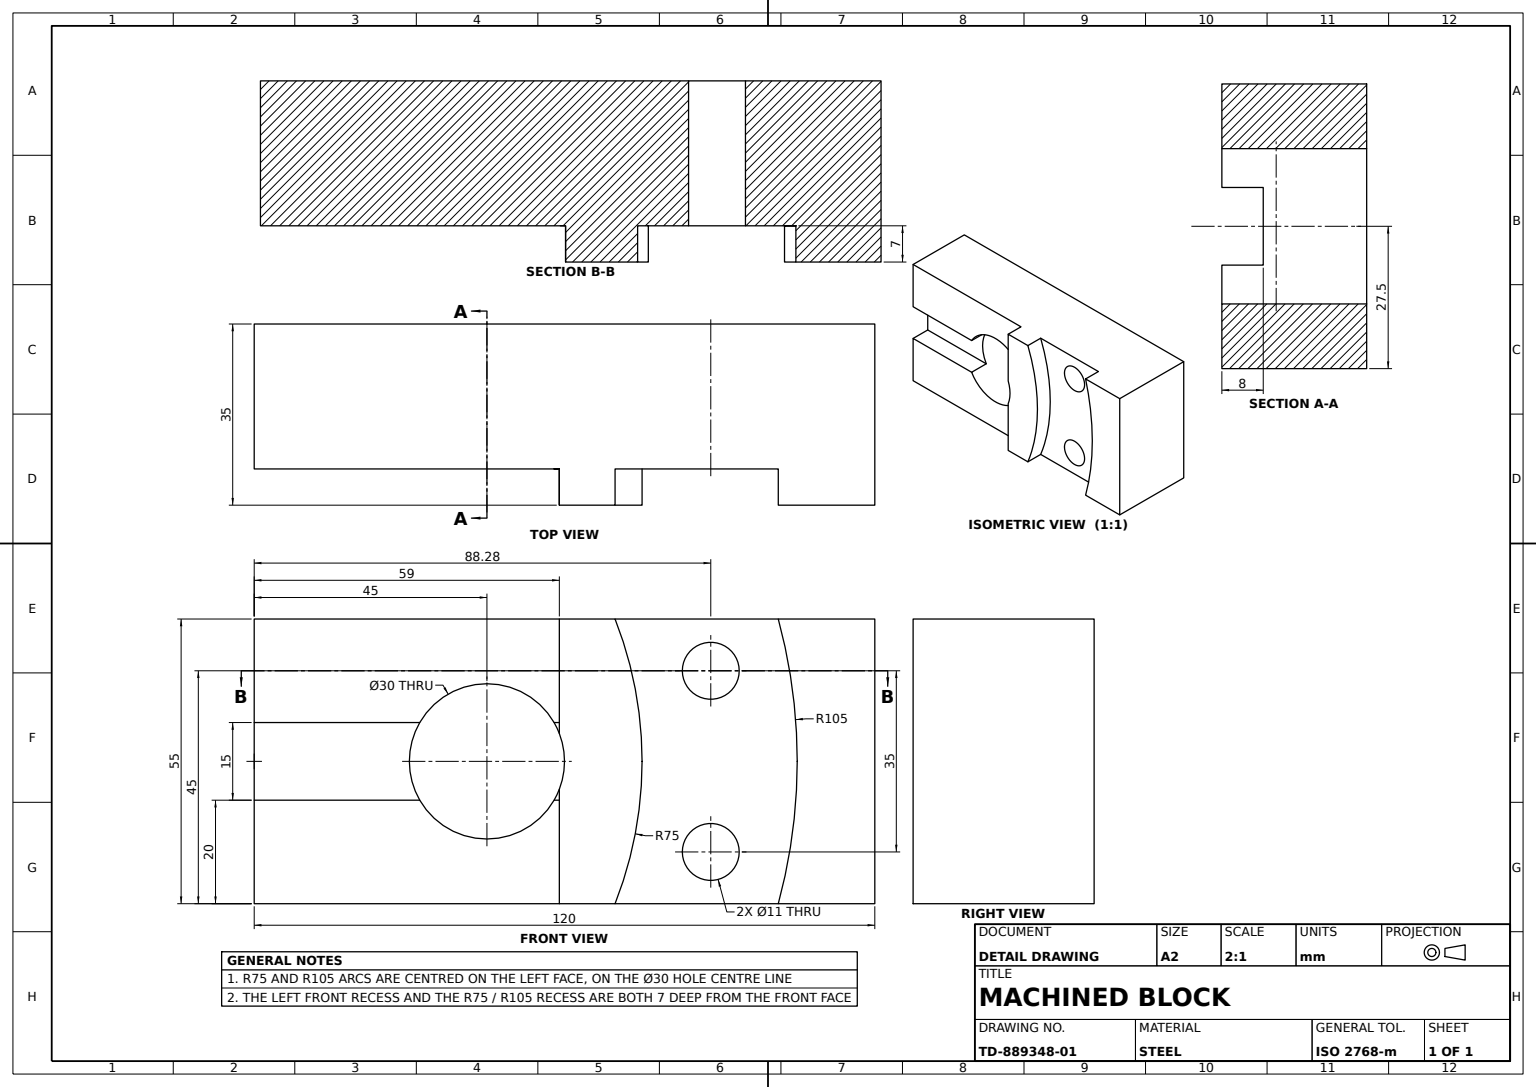
from build123d import *

# Parameters (mm, degrees)
SLIDE_PROFILE_SKETCH_W   = 120
SLIDE_PROFILE_SKETCH_H   = 55
SLIDE_PROFILE_SKETCH_R   = 15
SLIDE_PROFILE_SKETCH_R_2 = 5.5
SLIDE_BODY_35MM_DEPTH    = 35
FACE_RECESS_7MM_DEPTH    = 7
CURVED_POCKET_SKETCH_W   = 59
CURVED_POCKET_SKETCH_H   = 55
CURVED_POCKET_7MM_DEPTH  = 7
THROUGH_CUT_SKETCH_W     = 8
THROUGH_CUT_SKETCH_H     = 15
THROUGH_CUT_59MM_DEPTH   = 59


with BuildPart() as part:
    # Slide Profile Sketch → Slide Body 35mm (new body)
    with BuildSketch(Plane.XY):
        with Locations((0, 27.5)):
            Rectangle(SLIDE_PROFILE_SKETCH_W, SLIDE_PROFILE_SKETCH_H)
        with Locations((-15, 27.5)):
            Circle(SLIDE_PROFILE_SKETCH_R, mode=Mode.SUBTRACT)
        with Locations((28.282217915, 45)):
            Circle(SLIDE_PROFILE_SKETCH_R_2, mode=Mode.SUBTRACT)
        with Locations((28.282217915, 10)):
            Circle(SLIDE_PROFILE_SKETCH_R_2, mode=Mode.SUBTRACT)
    extrude(amount=SLIDE_BODY_35MM_DEPTH)

    # Face Recess Sketch → Face Recess 7mm (cut)
    with BuildSketch(Plane.XY.offset(35)):
        with BuildLine():
            Line((9.776428685, 55), (41.334840998, 55))
            ThreePointArc((41.334840998, 55), (45, 27.5), (41.334840998, 0))
            Line((41.334840998, 0), (9.776428685, 0))
            ThreePointArc((9.776428685, 0), (15, 27.5), (9.776428685, 55))
        make_face()
    extrude(amount=-FACE_RECESS_7MM_DEPTH, mode=Mode.SUBTRACT)

    # Curved Pocket Sketch → Curved Pocket 7mm (cut)
    with BuildSketch(Plane.XY.offset(35)):
        with Locations((-30.5, 27.5)):
            Rectangle(CURVED_POCKET_SKETCH_W, CURVED_POCKET_SKETCH_H)
    extrude(amount=-CURVED_POCKET_7MM_DEPTH, mode=Mode.SUBTRACT)

    # Through Cut Sketch → Through Cut 59mm (cut)
    with BuildSketch(Plane.ZY.offset(60)):
        with Locations((24, 27.5)):
            Rectangle(THROUGH_CUT_SKETCH_W, THROUGH_CUT_SKETCH_H)
    extrude(amount=-THROUGH_CUT_59MM_DEPTH, mode=Mode.SUBTRACT)


solid = part.part
